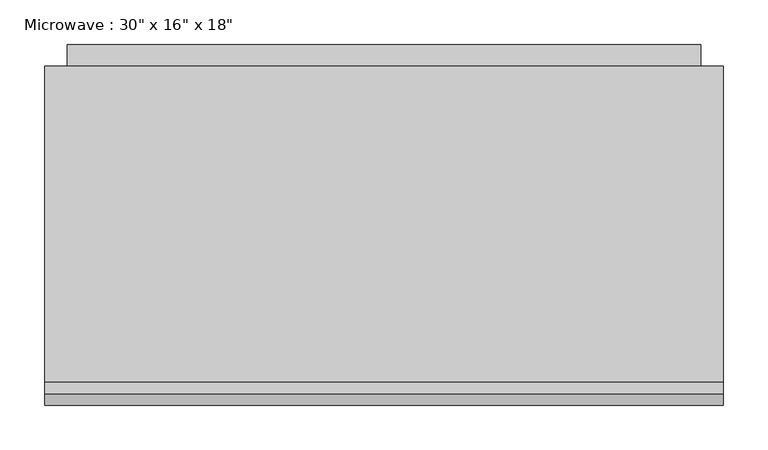
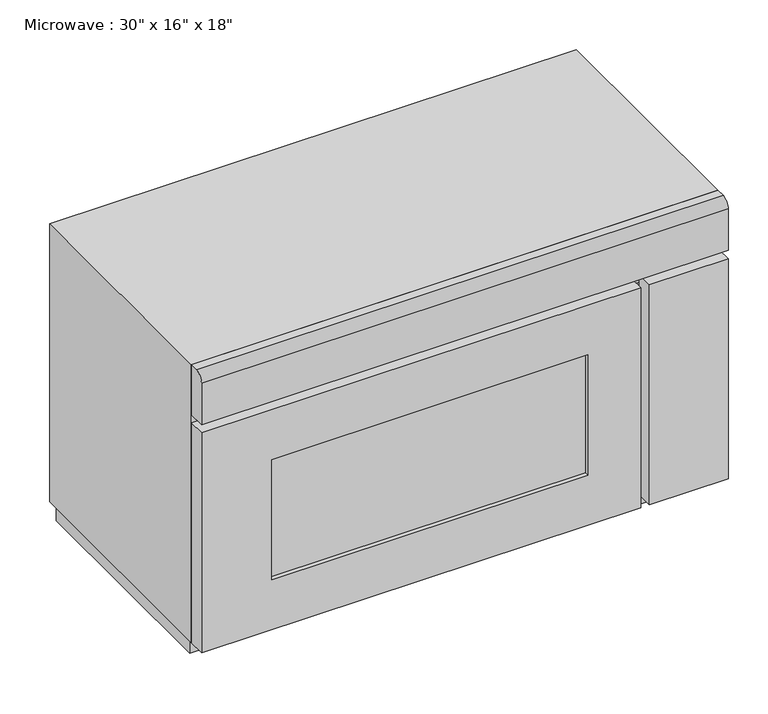
"""IFC4 building model written with IfcOpenShell, lengths in millimetres: proxy geometry."""

from ifc_helpers import new_model, si_unit, point, frame, frame_2d, origin, place, context, project, spatial, polyline, circle_curve, trimmed, segment, composite_curve, outline, extrude, faceted_brep, source, transform, mapped, element, save


def proxy_8a8d5ab2(model_context):
    return source(origin(), model_context, "Body", "SolidModel", [
        extrude(outline(polyline([(678.4897523, -549.9305058), (220.8928773, -549.9305058), (220.8928773, -543.5805058), (678.4897523, -543.5805058), (678.4897523, -549.9305058)])), frame((0.0, 0.0, 1022.35), z_axis=(0.0, 0.0, 1.0), x_axis=(1.0, 0.0, 0.0)), (0.0, 0.0, 1.0), 184.15),
        extrude(outline(polyline([(1282.7, 754.6897523), (1282.7, 119.2928773), (946.15, 119.2928773), (946.15, 754.6897523), (1282.7, 754.6897523)]), holes=[polyline([(1206.5, 678.4897523), (1022.35, 678.4897523), (1022.35, 220.8928773), (1206.5, 220.8928773), (1206.5, 678.4897523)])]), frame((0.0, -556.2805058, 0.0), z_axis=(0.0, 1.0, 0.0), x_axis=(0.0, 0.0, 1.0)), (0.0, 0.0, 1.0), 25.4),
        extrude(outline(polyline([(881.2928773, -556.2805058), (767.3897523, -556.2805058), (767.3897523, -530.8805058), (881.2928773, -530.8805058), (881.2928773, -556.2805058)])), frame((0.0, 0.0, 946.15), z_axis=(0.0, 0.0, 1.0), x_axis=(1.0, 0.0, 0.0)), (0.0, 0.0, 1.0), 336.55),
        extrude(outline(composite_curve([segment(polyline([(-543.5805058, 1371.6), (-530.8805058, 1371.6), (-530.8805058, 1295.4), (-556.2805058, 1295.4), (-556.2805058, 1358.9)]), True, "CONTINUOUS"), segment(trimmed(circle_curve(frame_2d((-543.5805058, 1358.9)), 12.7), [point((-556.2805058, 1358.9))], [point((-543.5805058, 1371.6))], False, "CARTESIAN"), True, "CONTINUOUS")], self_intersect=False)), frame((119.2928773, 0.0, 0.0), z_axis=(1.0, 0.0, 0.0), x_axis=(0.0, 1.0, 0.0)), (0.0, 0.0, 1.0), 762.0),
        extrude(outline(polyline([(-151.0441495, 1346.2), (-151.0441495, 961.946551), (-176.4441495, 936.546551), (-176.4441495, 1346.2), (-151.0441495, 1346.2)])), frame((144.6928773, 0.0, 0.0), z_axis=(1.0, 0.0, 0.0), x_axis=(0.0, 1.0, 0.0)), (0.0, 0.0, 1.0), 711.2),
        faceted_brep([(881.2928773, -175.2805058, 1371.6), (119.2928773, -175.2805058, 1371.6), (119.2928773, -530.8805058, 1371.6), (881.2928773, -530.8805058, 1371.6), (881.2928773, -175.2805058, 946.15), (881.2928773, -530.8805058, 946.15), (119.2928773, -530.8805058, 946.15), (119.2928773, -175.2805058, 946.15), (824.5397523, -530.8805058, 1271.0014904), (824.5397523, -530.8805058, 1020.1764904), (176.0460023, -530.8805058, 1020.1764904), (176.0460023, -530.8805058, 1271.0014904), (824.5397523, -200.6805058, 1271.0014904), (176.0460023, -200.6805058, 1271.0014904), (176.0460023, -200.6805058, 1020.1764904), (824.5397523, -200.6805058, 1020.1764904)], [[[0, 1, 2, 3]], [[4, 5, 6, 7]], [[1, 0, 4, 7]], [[2, 1, 7, 6]], [[3, 2, 6, 5], [8, 9, 10, 11]], [[0, 3, 5, 4]], [[12, 13, 14, 15]], [[12, 15, 9, 8]], [[15, 14, 10, 9]], [[14, 13, 11, 10]], [[13, 12, 8, 11]]]),
        extrude(outline(polyline([(871.7678773, -175.2805058), (871.7678773, -510.2430058), (128.8178773, -510.2430058), (128.8178773, -175.2805058), (871.7678773, -175.2805058)])), frame((0.0, 0.0, 914.4), z_axis=(0.0, 0.0, 1.0), x_axis=(1.0, 0.0, 0.0)), (0.0, 0.0, 1.0), 31.75),
    ])


if __name__ == "__main__":
    model = new_model("IFC4")
    model_context = context("Model", 3, world=origin())
    ifc_project = project(units=[si_unit("LENGTHUNIT", "METRE", prefix="MILLI")], contexts=[model_context])
    site = spatial("IfcSite", under=ifc_project)
    building = spatial("IfcBuilding", under=site)
    placement = place(None, origin())
    proxy_shape = proxy_8a8d5ab2(model_context)
    element("IfcBuildingElementProxy", 1, Name="Microwave : 30\" x 16\" x 18\"", ObjectType="Microwave : 30\" x 16\" x 18\"", at=placement, inside=building, context=model_context, shape_type="MappedRepresentation", body=[
        mapped(proxy_shape, transform((0.0, 0.0, 0.0), x_axis=(1.0, 0.0, 0.0), y_axis=(0.0, 1.0, 0.0), z_axis=(0.0, 0.0, 1.0))),
    ])
    save(model, "model.ifc")

# Revit data of these elements
# Type "Microwave : 30\" x 16\" x 18\""
#   Assembly Code = "E1090400"
#   Depth = 1' - 4"
#   Height = 1' - 6"
#   Width = 2' - 6"
#   Microwave Material = Laminate - Ivory, Glossy
#   Default Elevation = 0
# Element 1 (IfcBuildingElementProxy, "Microwave : 30\" x 16\" x 18\"")
#   Materials on its faces: "Laminate - Ivory, Glossy", "Glass"
# Materials
#   "Laminate - Ivory, Glossy": colour RGB 247 247 239, transparency 0
#   "Glass": class "Glass", colour RGB 0 128 192, transparency 0.75, Description = "Soda Lime Glass", Cost = 0
